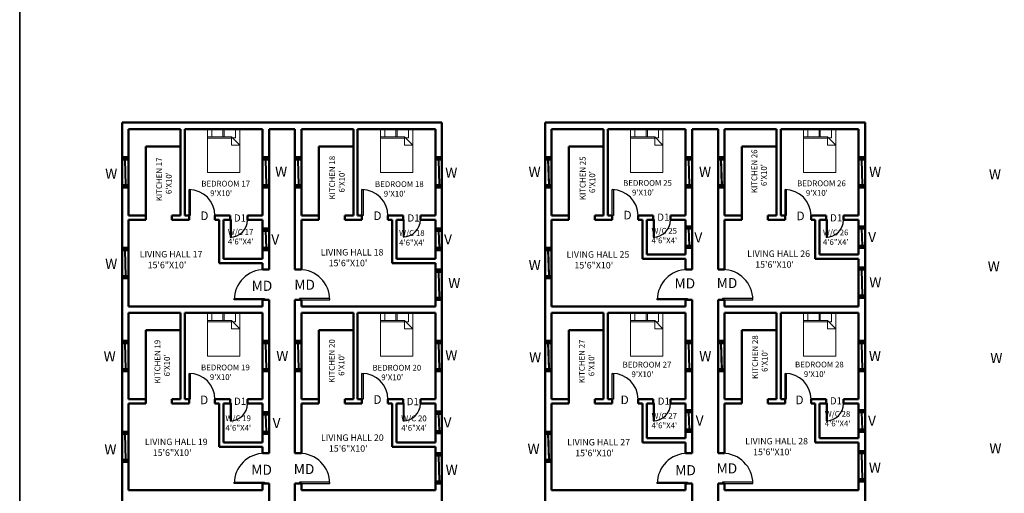
# Model space of a CAD drawing. Units: inches. Extents: x 9239 to 26065, y 6728 to 14611.
# Tile 8 of 12: x 23324 to 24691, y 12444 to 13102. Entities that reach past the tile are written whole.
import ezdxf

# ---------------------------------------------------------------- set-up
doc = ezdxf.new("R2010")
doc.units = ezdxf.units.IN
doc.header["$MEASUREMENT"] = 0
for name, color, linetype, lineweight in [('A-ANNO-TEXT', 7, 'Continuous', 18), ('A-ANNO-TTLB', 7, 'Continuous', 35), ('A-AREA-IDEN', 7, 'Continuous', 18), ('A-DOOR', 4, 'Continuous', 25), ('A-FURN', 8, 'Continuous', 18), ('A-GLAZ', 4, 'Continuous', 25), ('A-WALL', 7, 'Continuous', 50)]:
    doc.layers.add(name, color=color, linetype=linetype, lineweight=lineweight)
doc.styles.get("Standard").update_dxf_attribs({"font": 'arial.ttf'})

# ---------------------------------------------------------------- blocks, each defined once
blk = doc.blocks.new('*U10')
for p, q in [((0, 0), (0, -6)), ((36, 0), (36, -6))]:
    blk.add_line(p, q)
blk.add_lwpolyline([(0, 0), (0, 36), (1.75, 36), (1.75, 0)], close=True)
blk.add_arc((0, 0), 36, 0, 90)
blk = doc.blocks.new('*U34')
for p, q in [((0, 0), (0, 6)), ((24, 0), (24, 6))]:
    blk.add_line(p, q)
blk.add_lwpolyline([(0, 0), (0, -24), (1.75, -24), (1.75, 0)], close=True)
blk.add_arc((0, 0), 24, 270, 0)
blk = doc.blocks.new('*U33')
for p, q in [((-40, 0), (-40, 6)), ((0, 0), (0, 6))]:
    blk.add_line(p, q)
blk.add_lwpolyline([(0, 0), (0, -40), (-1.75, -40), (-1.75, 0)], close=True)
blk.add_arc((0, 0), 40, 180, 270)
blk = doc.blocks.new('*U35')
for p, q in [((0, 0), (0, -6)), ((-40, 0), (-40, -6))]:
    blk.add_line(p, q)
blk.add_lwpolyline([(0, 0), (0, 40), (-1.75, 40), (-1.75, 0)], close=True)
blk.add_arc((0, 0), 40, 90, 180)
blk = doc.blocks.new('Bed - Queen')
for p, q in [((0, -80.00003), (0, 0)), ((0, 0), (59.99999, 0)), ((59.99999, 0), (59.99999, -80.00003)), ((0, -14.4), (44.8, -14.4)), ((44.8, -16.8), (0, -16.8)), ((7.99999, -1.2), (28.79998, -1.2)), ((7.99999, -14.4), (7.99999, -1.2)), ((28.79998, -1.2), (28.79998, -14.4)), ((31.19999, -1.2), (51.99999, -1.2)), ((31.19999, -14.4), (31.19999, -1.2)), ((59.99999, -29.6), (44.8, -14.4)), ((44.8, -14.4), (44.8, -29.6)), ((51.99999, -16.4), (46.79936, -16.4)), ((51.99999, -1.2), (51.99999, -16.4)), ((44.8, -29.6), (59.99999, -29.6)), ((59.99999, -80.00003), (0, -80.00003))]:
    blk.add_line(p, q)
blk = doc.blocks.new('WIN-36')
for p, q in [((0, 1), (36, 1)), ((0, 0.5), (36, 0.5)), ((0, 0), (36, 0))]:
    blk.add_line(p, q)
blk = doc.blocks.new('WIN-24')
for p, q in [((0, 1), (24, 1)), ((0, 0.5), (24, 0.5)), ((0, 0), (24, 0))]:
    blk.add_line(p, q)

msp = doc.modelspace()

# ---------------------------------------------------------------- linework, layer by layer
at = {"layer": 'A-ANNO-TTLB'}
msp.add_lwpolyline([(23324.14, 14611.25), (26064.6, 14611.25), (26064.6, 11591.84), (23324.14, 11591.84)], close=True, dxfattribs=at)
at = {"layer": 'A-WALL'}
for p, q in [((23466.16, 12958.64), (23910.16, 12958.64)), ((23466.16, 11854.64), (23466.16, 12958.64)), ((23910.16, 12958.64), (23910.16, 11854.64)), ((24053.28, 12958.64), (24497.28, 12958.64)), ((24053.28, 11854.64), (24053.28, 12958.64)), ((24497.28, 12958.64), (24497.28, 11854.64)), ((23475.16, 12949.64), (23547.16, 12949.64)), ((23475.16, 12829.64), (23475.16, 12949.64)), ((23547.16, 12829.64), (23547.16, 12949.64)), ((23553.16, 12829.64), (23553.16, 12949.64)), ((23553.16, 12949.64), (23661.16, 12949.64)), ((23661.16, 12829.64), (23661.16, 12949.64)), ((23670.16, 12754.64), (23670.16, 12949.64)), ((23670.16, 12949.64), (23706.16, 12949.64)), ((23706.16, 12949.64), (23706.16, 12754.64)), ((23715.16, 12949.64), (23715.16, 12829.64)), ((23715.16, 12949.64), (23787.16, 12949.64)), ((23787.16, 12949.64), (23787.16, 12829.64)), ((23793.16, 12949.64), (23793.16, 12829.64)), ((23793.16, 12949.64), (23901.16, 12949.64)), ((23901.16, 12949.64), (23901.16, 12829.64)), ((24062.28, 12949.64), (24134.28, 12949.64)), ((24062.28, 12829.64), (24062.28, 12949.64)), ((24134.28, 12829.64), (24134.28, 12949.64)), ((24140.28, 12829.64), (24140.28, 12949.64)), ((24140.28, 12949.64), (24248.28, 12949.64)), ((24248.28, 12829.64), (24248.28, 12949.64)), ((24257.28, 12754.64), (24257.28, 12949.64)), ((24257.28, 12949.64), (24293.28, 12949.64)), ((24293.28, 12949.64), (24293.28, 12754.64)), ((24302.28, 12949.64), (24302.28, 12829.64)), ((24302.28, 12949.64), (24374.28, 12949.64)), ((24374.28, 12949.64), (24374.28, 12829.64)), ((24380.28, 12949.64), (24380.28, 12829.64)), ((24380.28, 12949.64), (24488.28, 12949.64)), ((24488.28, 12949.64), (24488.28, 12829.64)), ((23499.16, 12829.64), (23499.16, 12925.64)), ((23499.16, 12925.64), (23547.16, 12925.64)), ((23739.16, 12925.64), (23739.16, 12829.64)), ((23739.16, 12925.64), (23787.16, 12925.64)), ((24086.28, 12829.64), (24086.28, 12925.64)), ((24086.28, 12925.64), (24134.28, 12925.64)), ((24326.28, 12925.64), (24326.28, 12829.64)), ((24326.28, 12925.64), (24374.28, 12925.64)), ((23475.16, 12910.64), (23466.16, 12910.64)), ((23475.16, 12907.64), (23466.16, 12907.64)), ((23661.16, 12910.64), (23670.16, 12910.64)), ((23661.16, 12907.64), (23670.16, 12907.64)), ((23715.16, 12910.64), (23706.16, 12910.64)), ((23715.16, 12907.64), (23706.16, 12907.64)), ((23901.16, 12910.64), (23910.16, 12910.64)), ((23901.16, 12907.64), (23910.16, 12907.64)), ((24062.28, 12910.64), (24053.28, 12910.64)), ((24062.28, 12907.64), (24053.28, 12907.64)), ((24248.28, 12910.64), (24257.28, 12910.64)), ((24248.28, 12907.64), (24257.28, 12907.64)), ((24302.28, 12910.64), (24293.28, 12910.64)), ((24302.28, 12907.64), (24293.28, 12907.64)), ((24488.28, 12910.64), (24497.28, 12910.64)), ((24488.28, 12907.64), (24497.28, 12907.64)), ((23475.16, 12871.64), (23466.16, 12871.64)), ((23661.16, 12871.64), (23670.16, 12871.64)), ((23715.16, 12871.64), (23706.16, 12871.64)), ((23901.16, 12871.64), (23910.16, 12871.64)), ((24062.28, 12871.64), (24053.28, 12871.64)), ((24248.28, 12871.64), (24257.28, 12871.64)), ((24302.28, 12871.64), (24293.28, 12871.64)), ((24488.28, 12871.64), (24497.28, 12871.64)), ((23475.16, 12868.64), (23466.16, 12868.64)), ((23661.16, 12868.64), (23670.16, 12868.64)), ((23715.16, 12868.64), (23706.16, 12868.64)), ((23901.16, 12868.64), (23910.16, 12868.64)), ((24062.28, 12868.64), (24053.28, 12868.64)), ((24248.28, 12868.64), (24257.28, 12868.64)), ((24302.28, 12868.64), (24293.28, 12868.64)), ((24488.28, 12868.64), (24497.28, 12868.64)), ((23475.16, 12829.64), (23499.16, 12829.64)), ((23475.16, 12823.64), (23499.16, 12823.64)), ((23475.16, 12703.64), (23475.16, 12823.64)), ((23499.16, 12823.64), (23499.16, 12829.64)), ((23535.16, 12823.64), (23535.16, 12829.64)), ((23535.16, 12829.64), (23547.16, 12829.64)), ((23535.16, 12823.64), (23559.16, 12823.64)), ((23553.16, 12829.64), (23559.16, 12829.64)), ((23559.16, 12823.64), (23559.16, 12829.64)), ((23595.16, 12823.64), (23595.16, 12829.64)), ((23595.16, 12829.64), (23616.16, 12829.64)), ((23595.16, 12823.64), (23601.16, 12823.64)), ((23601.16, 12763.64), (23601.16, 12823.64)), ((23607.16, 12769.64), (23607.16, 12823.64)), ((23607.16, 12823.64), (23616.16, 12823.64)), ((23616.16, 12823.64), (23616.16, 12829.64)), ((23640.16, 12823.64), (23640.16, 12829.64)), ((23640.16, 12829.64), (23661.16, 12829.64)), ((23640.16, 12823.64), (23661.16, 12823.64)), ((23661.16, 12769.64), (23661.16, 12823.64)), ((23715.16, 12829.64), (23739.16, 12829.64)), ((23715.16, 12823.64), (23739.16, 12823.64)), ((23715.16, 12823.64), (23715.16, 12754.64)), ((23739.16, 12829.64), (23739.16, 12823.64)), ((23775.16, 12829.64), (23775.16, 12823.64)), ((23775.16, 12829.64), (23787.16, 12829.64)), ((23775.16, 12823.64), (23799.16, 12823.64)), ((23793.16, 12829.64), (23799.16, 12829.64)), ((23799.16, 12829.64), (23799.16, 12823.64)), ((23835.16, 12829.64), (23835.16, 12823.64)), ((23835.16, 12829.64), (23856.16, 12829.64)), ((23835.16, 12823.64), (23841.16, 12823.64)), ((23841.16, 12823.64), (23841.16, 12763.64)), ((23847.16, 12823.64), (23847.16, 12769.64)), ((23847.16, 12823.64), (23856.16, 12823.64)), ((23856.16, 12829.64), (23856.16, 12823.64)), ((23880.16, 12829.64), (23880.16, 12823.64)), ((23880.16, 12829.64), (23901.16, 12829.64)), ((23880.16, 12823.64), (23901.16, 12823.64)), ((23901.16, 12823.64), (23901.16, 12769.64)), ((24062.28, 12829.64), (24086.28, 12829.64)), ((24062.28, 12823.64), (24086.28, 12823.64)), ((24062.28, 12703.64), (24062.28, 12823.64)), ((24086.28, 12823.64), (24086.28, 12829.64)), ((24122.28, 12823.64), (24122.28, 12829.64)), ((24122.28, 12829.64), (24134.28, 12829.64)), ((24122.28, 12823.64), (24146.28, 12823.64)), ((24140.28, 12829.64), (24146.28, 12829.64)), ((24146.28, 12823.64), (24146.28, 12829.64)), ((24182.28, 12823.64), (24182.28, 12829.64)), ((24182.28, 12829.64), (24203.28, 12829.64)), ((24182.28, 12823.64), (24188.28, 12823.64)), ((24188.28, 12769.64), (24188.28, 12823.64)), ((24194.28, 12775.64), (24194.28, 12823.64)), ((24194.28, 12823.64), (24203.28, 12823.64)), ((24203.28, 12823.64), (24203.28, 12829.64)), ((24227.28, 12823.64), (24227.28, 12829.64)), ((24227.28, 12829.64), (24248.28, 12829.64)), ((24227.28, 12823.64), (24248.28, 12823.64)), ((24248.28, 12775.64), (24248.28, 12823.64)), ((24302.28, 12829.64), (24326.28, 12829.64)), ((24302.28, 12823.64), (24326.28, 12823.64)), ((24302.28, 12823.64), (24302.28, 12754.64)), ((24326.28, 12829.64), (24326.28, 12823.64)), ((24362.28, 12829.64), (24362.28, 12823.64)), ((24362.28, 12829.64), (24374.28, 12829.64)), ((24362.28, 12823.64), (24386.28, 12823.64)), ((24380.28, 12829.64), (24386.28, 12829.64)), ((24386.28, 12829.64), (24386.28, 12823.64)), ((24422.28, 12829.64), (24422.28, 12823.64)), ((24422.28, 12829.64), (24443.28, 12829.64)), ((24422.28, 12823.64), (24428.28, 12823.64)), ((24428.28, 12823.64), (24428.28, 12769.64)), ((24434.28, 12823.64), (24434.28, 12775.64)), ((24434.28, 12823.64), (24443.28, 12823.64)), ((24443.28, 12829.64), (24443.28, 12823.64)), ((24467.28, 12829.64), (24467.28, 12823.64)), ((24467.28, 12829.64), (24488.28, 12829.64)), ((24467.28, 12823.64), (24488.28, 12823.64)), ((24488.28, 12823.64), (24488.28, 12775.64)), ((23661.16, 12811.64), (23670.16, 12811.64)), ((23661.16, 12808.64), (23670.16, 12808.64)), ((23901.16, 12811.64), (23910.16, 12811.64)), ((23901.16, 12808.64), (23910.16, 12808.64)), ((24248.28, 12814.64), (24257.28, 12814.64)), ((24248.28, 12811.64), (24257.28, 12811.64)), ((24488.28, 12814.64), (24497.28, 12814.64)), ((24488.28, 12811.64), (24497.28, 12811.64)), ((23475.16, 12784.64), (23466.16, 12784.64)), ((23475.16, 12781.64), (23466.16, 12781.64)), ((23661.16, 12784.64), (23670.16, 12784.64)), ((23661.16, 12781.64), (23670.16, 12781.64)), ((23901.16, 12784.64), (23910.16, 12784.64)), ((23901.16, 12781.64), (23910.16, 12781.64)), ((24062.28, 12784.64), (24053.28, 12784.64)), ((24062.28, 12781.64), (24053.28, 12781.64)), ((24248.28, 12787.64), (24257.28, 12787.64)), ((24248.28, 12784.64), (24257.28, 12784.64)), ((24488.28, 12787.64), (24497.28, 12787.64)), ((24488.28, 12784.64), (24497.28, 12784.64)), ((23601.16, 12763.64), (23661.16, 12763.64)), ((23607.16, 12769.64), (23661.16, 12769.64)), ((23661.16, 12754.64), (23661.16, 12763.64)), ((23841.16, 12763.64), (23901.16, 12763.64)), ((23847.16, 12769.64), (23901.16, 12769.64)), ((23901.16, 12763.64), (23901.16, 12703.64)), ((24188.28, 12769.64), (24248.28, 12769.64)), ((24194.28, 12775.64), (24248.28, 12775.64)), ((24248.28, 12754.64), (24248.28, 12769.64)), ((24428.28, 12769.64), (24488.28, 12769.64)), ((24434.28, 12775.64), (24488.28, 12775.64)), ((24488.28, 12769.64), (24488.28, 12703.64)), ((23661.16, 12754.64), (23670.16, 12754.64)), ((23706.16, 12754.64), (23715.16, 12754.64)), ((23901.16, 12754.64), (23910.16, 12754.64)), ((23901.16, 12751.64), (23910.16, 12751.64)), ((24248.28, 12754.64), (24257.28, 12754.64)), ((24293.28, 12754.64), (24302.28, 12754.64)), ((24488.28, 12757.64), (24497.28, 12757.64)), ((24488.28, 12754.64), (24497.28, 12754.64)), ((23475.16, 12745.64), (23466.16, 12745.64)), ((23475.16, 12742.64), (23466.16, 12742.64)), ((24062.28, 12745.64), (24053.28, 12745.64)), ((24062.28, 12742.64), (24053.28, 12742.64)), ((23661.16, 12712.64), (23670.16, 12712.64)), ((23661.16, 12703.64), (23661.16, 12712.64)), ((23670.16, 12499.64), (23670.16, 12712.64)), ((23706.16, 12712.64), (23715.16, 12712.64)), ((23706.16, 12712.64), (23706.16, 12499.64)), ((23715.16, 12712.64), (23715.16, 12703.64)), ((23901.16, 12715.64), (23910.16, 12715.64)), ((23901.16, 12712.64), (23910.16, 12712.64)), ((24248.28, 12712.64), (24257.28, 12712.64)), ((24248.28, 12703.64), (24248.28, 12712.64)), ((24257.28, 12499.64), (24257.28, 12712.64)), ((24293.28, 12712.64), (24302.28, 12712.64)), ((24293.28, 12712.64), (24293.28, 12499.64)), ((24302.28, 12712.64), (24302.28, 12703.64)), ((24488.28, 12718.64), (24497.28, 12718.64)), ((24488.28, 12715.64), (24497.28, 12715.64)), ((23475.16, 12703.64), (23661.16, 12703.64)), ((23475.16, 12694.64), (23547.16, 12694.64)), ((23475.16, 12574.64), (23475.16, 12694.64)), ((23547.16, 12574.64), (23547.16, 12694.64)), ((23553.16, 12574.64), (23553.16, 12694.64)), ((23553.16, 12694.64), (23661.16, 12694.64)), ((23661.16, 12574.64), (23661.16, 12694.64)), ((23715.16, 12703.64), (23901.16, 12703.64)), ((23715.16, 12694.64), (23787.16, 12694.64)), ((23715.16, 12694.64), (23715.16, 12574.64)), ((23787.16, 12694.64), (23787.16, 12574.64)), ((23793.16, 12694.64), (23793.16, 12574.64)), ((23793.16, 12694.64), (23901.16, 12694.64)), ((23901.16, 12694.64), (23901.16, 12574.64)), ((24062.28, 12703.64), (24248.28, 12703.64)), ((24062.28, 12694.64), (24134.28, 12694.64)), ((24062.28, 12574.64), (24062.28, 12694.64)), ((24134.28, 12574.64), (24134.28, 12694.64)), ((24140.28, 12574.64), (24140.28, 12694.64)), ((24140.28, 12694.64), (24248.28, 12694.64)), ((24248.28, 12574.64), (24248.28, 12694.64)), ((24302.28, 12703.64), (24488.28, 12703.64)), ((24302.28, 12694.64), (24374.28, 12694.64)), ((24302.28, 12694.64), (24302.28, 12574.64)), ((24374.28, 12694.64), (24374.28, 12574.64)), ((24380.28, 12694.64), (24380.28, 12574.64)), ((24380.28, 12694.64), (24488.28, 12694.64)), ((24488.28, 12694.64), (24488.28, 12574.64)), ((23499.16, 12574.64), (23499.16, 12670.64)), ((23499.16, 12670.64), (23547.16, 12670.64)), ((23739.16, 12670.64), (23739.16, 12574.64)), ((23739.16, 12670.64), (23787.16, 12670.64)), ((24086.28, 12574.64), (24086.28, 12670.64)), ((24086.28, 12670.64), (24134.28, 12670.64)), ((24326.28, 12670.64), (24326.28, 12574.64)), ((24326.28, 12670.64), (24374.28, 12670.64)), ((23475.16, 12655.64), (23466.16, 12655.64)), ((23661.16, 12655.64), (23670.16, 12655.64)), ((23715.16, 12655.64), (23706.16, 12655.64)), ((23901.16, 12655.64), (23910.16, 12655.64)), ((24062.28, 12655.64), (24053.28, 12655.64)), ((24248.28, 12655.64), (24257.28, 12655.64)), ((24302.28, 12655.64), (24293.28, 12655.64)), ((24488.28, 12655.64), (24497.28, 12655.64)), ((23475.16, 12652.64), (23466.16, 12652.64)), ((23661.16, 12652.64), (23670.16, 12652.64)), ((23715.16, 12652.64), (23706.16, 12652.64)), ((23901.16, 12652.64), (23910.16, 12652.64)), ((24062.28, 12652.64), (24053.28, 12652.64)), ((24248.28, 12652.64), (24257.28, 12652.64)), ((24302.28, 12652.64), (24293.28, 12652.64)), ((24488.28, 12652.64), (24497.28, 12652.64)), ((23475.16, 12616.64), (23466.16, 12616.64)), ((23475.16, 12613.64), (23466.16, 12613.64)), ((23661.16, 12616.64), (23670.16, 12616.64)), ((23661.16, 12613.64), (23670.16, 12613.64)), ((23715.16, 12616.64), (23706.16, 12616.64)), ((23715.16, 12613.64), (23706.16, 12613.64)), ((23901.16, 12616.64), (23910.16, 12616.64)), ((23901.16, 12613.64), (23910.16, 12613.64)), ((24062.28, 12616.64), (24053.28, 12616.64)), ((24062.28, 12613.64), (24053.28, 12613.64)), ((24248.28, 12616.64), (24257.28, 12616.64)), ((24248.28, 12613.64), (24257.28, 12613.64)), ((24302.28, 12616.64), (24293.28, 12616.64)), ((24302.28, 12613.64), (24293.28, 12613.64)), ((24488.28, 12616.64), (24497.28, 12616.64)), ((24488.28, 12613.64), (24497.28, 12613.64)), ((23475.16, 12574.64), (23499.16, 12574.64)), ((23499.16, 12568.64), (23499.16, 12574.64)), ((23535.16, 12568.64), (23535.16, 12574.64)), ((23535.16, 12574.64), (23547.16, 12574.64)), ((23553.16, 12574.64), (23559.16, 12574.64)), ((23559.16, 12568.64), (23559.16, 12574.64)), ((23595.16, 12568.64), (23595.16, 12574.64)), ((23595.16, 12574.64), (23616.16, 12574.64)), ((23616.16, 12568.64), (23616.16, 12574.64)), ((23640.16, 12568.64), (23640.16, 12574.64)), ((23640.16, 12574.64), (23661.16, 12574.64)), ((23715.16, 12574.64), (23739.16, 12574.64)), ((23739.16, 12574.64), (23739.16, 12568.64)), ((23775.16, 12574.64), (23775.16, 12568.64)), ((23775.16, 12574.64), (23787.16, 12574.64)), ((23793.16, 12574.64), (23799.16, 12574.64)), ((23799.16, 12574.64), (23799.16, 12568.64)), ((23835.16, 12574.64), (23835.16, 12568.64)), ((23835.16, 12574.64), (23856.16, 12574.64)), ((23856.16, 12574.64), (23856.16, 12568.64)), ((23880.16, 12574.64), (23880.16, 12568.64)), ((23880.16, 12574.64), (23901.16, 12574.64)), ((24062.28, 12574.64), (24086.28, 12574.64)), ((24086.28, 12568.64), (24086.28, 12574.64)), ((24122.28, 12568.64), (24122.28, 12574.64)), ((24122.28, 12574.64), (24134.28, 12574.64)), ((24140.28, 12574.64), (24146.28, 12574.64)), ((24146.28, 12568.64), (24146.28, 12574.64)), ((24182.28, 12568.64), (24182.28, 12574.64)), ((24182.28, 12574.64), (24203.28, 12574.64)), ((24203.28, 12568.64), (24203.28, 12574.64)), ((24227.28, 12568.64), (24227.28, 12574.64)), ((24227.28, 12574.64), (24248.28, 12574.64)), ((24302.28, 12574.64), (24326.28, 12574.64)), ((24326.28, 12574.64), (24326.28, 12568.64)), ((24362.28, 12574.64), (24362.28, 12568.64)), ((24362.28, 12574.64), (24374.28, 12574.64)), ((24380.28, 12574.64), (24386.28, 12574.64)), ((24386.28, 12574.64), (24386.28, 12568.64)), ((24422.28, 12574.64), (24422.28, 12568.64)), ((24422.28, 12574.64), (24443.28, 12574.64)), ((24443.28, 12574.64), (24443.28, 12568.64)), ((24467.28, 12574.64), (24467.28, 12568.64)), ((24467.28, 12574.64), (24488.28, 12574.64)), ((23475.16, 12568.64), (23499.16, 12568.64)), ((23475.16, 12448.64), (23475.16, 12568.64)), ((23535.16, 12568.64), (23559.16, 12568.64)), ((23595.16, 12568.64), (23601.16, 12568.64)), ((23601.16, 12508.64), (23601.16, 12568.64)), ((23607.16, 12514.64), (23607.16, 12568.64)), ((23607.16, 12568.64), (23616.16, 12568.64)), ((23640.16, 12568.64), (23661.16, 12568.64)), ((23661.16, 12514.64), (23661.16, 12568.64)), ((23715.16, 12568.64), (23739.16, 12568.64)), ((23715.16, 12568.64), (23715.16, 12499.64)), ((23775.16, 12568.64), (23799.16, 12568.64)), ((23835.16, 12568.64), (23841.16, 12568.64)), ((23841.16, 12568.64), (23841.16, 12508.64)), ((23847.16, 12568.64), (23847.16, 12514.64)), ((23847.16, 12568.64), (23856.16, 12568.64)), ((23880.16, 12568.64), (23901.16, 12568.64)), ((23901.16, 12568.64), (23901.16, 12514.64)), ((23901.16, 12557.55), (23910.16, 12557.55)), ((24062.28, 12568.64), (24086.28, 12568.64)), ((24062.28, 12448.64), (24062.28, 12568.64)), ((24122.28, 12568.64), (24146.28, 12568.64)), ((24182.28, 12568.64), (24188.28, 12568.64)), ((24188.28, 12514.64), (24188.28, 12568.64)), ((24194.28, 12520.64), (24194.28, 12568.64)), ((24194.28, 12568.64), (24203.28, 12568.64)), ((24227.28, 12568.64), (24248.28, 12568.64)), ((24248.28, 12520.64), (24248.28, 12568.64)), ((24248.28, 12559.64), (24257.28, 12559.64)), ((24302.28, 12568.64), (24326.28, 12568.64)), ((24302.28, 12568.64), (24302.28, 12499.64)), ((24362.28, 12568.64), (24386.28, 12568.64)), ((24422.28, 12568.64), (24428.28, 12568.64)), ((24428.28, 12568.64), (24428.28, 12514.64)), ((24434.28, 12568.64), (24434.28, 12520.64)), ((24434.28, 12568.64), (24443.28, 12568.64)), ((24467.28, 12568.64), (24488.28, 12568.64)), ((24488.28, 12568.64), (24488.28, 12520.64)), ((24488.28, 12559.64), (24497.28, 12559.64)), ((23661.16, 12556.64), (23670.16, 12556.64)), ((23661.16, 12553.64), (23670.16, 12553.64)), ((23901.16, 12554.55), (23910.16, 12554.55)), ((24248.28, 12556.64), (24257.28, 12556.64)), ((24488.28, 12556.64), (24497.28, 12556.64)), ((23901.16, 12530.55), (23910.16, 12530.55)), ((24248.28, 12532.64), (24257.28, 12532.64)), ((24488.28, 12532.64), (24497.28, 12532.64)), ((23475.16, 12529.64), (23466.16, 12529.64)), ((23475.16, 12526.64), (23466.16, 12526.64)), ((23661.16, 12529.64), (23670.16, 12529.64)), ((23661.16, 12526.64), (23670.16, 12526.64)), ((23901.16, 12527.55), (23910.16, 12527.55)), ((24062.28, 12529.64), (24053.28, 12529.64)), ((24062.28, 12526.64), (24053.28, 12526.64)), ((24194.28, 12520.64), (24248.28, 12520.64)), ((24248.28, 12529.64), (24257.28, 12529.64)), ((24434.28, 12520.64), (24488.28, 12520.64)), ((24488.28, 12529.64), (24497.28, 12529.64)), ((23601.16, 12508.64), (23661.16, 12508.64)), ((23607.16, 12514.64), (23661.16, 12514.64)), ((23661.16, 12499.64), (23661.16, 12508.64)), ((23841.16, 12508.64), (23901.16, 12508.64)), ((23847.16, 12514.64), (23901.16, 12514.64)), ((23901.16, 12508.64), (23901.16, 12448.64)), ((24188.28, 12514.64), (24248.28, 12514.64)), ((24248.28, 12499.64), (24248.28, 12514.64)), ((24428.28, 12514.64), (24488.28, 12514.64)), ((24488.28, 12514.64), (24488.28, 12448.64)), ((24488.28, 12502.64), (24497.28, 12502.64)), ((23475.16, 12490.64), (23466.16, 12490.64)), ((23661.16, 12499.64), (23670.16, 12499.64)), ((23706.16, 12499.64), (23715.16, 12499.64)), ((23901.16, 12499.64), (23910.16, 12499.64)), ((23901.16, 12496.64), (23910.16, 12496.64)), ((24062.28, 12490.64), (24053.28, 12490.64)), ((24248.28, 12499.64), (24257.28, 12499.64)), ((24293.28, 12499.64), (24302.28, 12499.64)), ((24488.28, 12499.64), (24497.28, 12499.64)), ((23475.16, 12487.64), (23466.16, 12487.64)), ((24062.28, 12487.64), (24053.28, 12487.64)), ((24488.28, 12463.64), (24497.28, 12463.64)), ((23475.16, 12448.64), (23661.16, 12448.64)), ((23661.16, 12457.64), (23670.16, 12457.64)), ((23661.16, 12448.64), (23661.16, 12457.64)), ((23670.16, 12244.64), (23670.16, 12457.64)), ((23706.16, 12457.64), (23715.16, 12457.64)), ((23706.16, 12457.64), (23706.16, 12244.64)), ((23715.16, 12457.64), (23715.16, 12448.64)), ((23715.16, 12448.64), (23901.16, 12448.64)), ((23901.16, 12460.64), (23910.16, 12460.64)), ((23901.16, 12457.64), (23910.16, 12457.64)), ((24062.28, 12448.64), (24248.28, 12448.64)), ((24248.28, 12457.64), (24257.28, 12457.64)), ((24248.28, 12448.64), (24248.28, 12457.64)), ((24257.28, 12244.64), (24257.28, 12457.64)), ((24293.28, 12457.64), (24302.28, 12457.64)), ((24293.28, 12457.64), (24293.28, 12244.64)), ((24302.28, 12457.64), (24302.28, 12448.64)), ((24302.28, 12448.64), (24488.28, 12448.64)), ((24488.28, 12460.64), (24497.28, 12460.64))]:
    msp.add_line(p, q, dxfattribs=at)

# ---------------------------------------------------------------- block references
at = {"layer": 'A-DOOR'}
for name, p in [('*U10', (23559.16, 12829.64)), ('*U10', (23799.16, 12829.64)), ('*U10', (24146.28, 12829.64)), ('*U10', (24386.28, 12829.64)), ('*U34', (23616.16, 12823.64)), ('*U34', (23856.16, 12823.97)), ('*U34', (24203.28, 12823.64)), ('*U34', (24443.28, 12823.64)), ('*U10', (23559.16, 12574.64)), ('*U10', (23799.16, 12574.64)), ('*U10', (24146.28, 12574.64)), ('*U10', (24386.28, 12574.64)), ('*U34', (23616.16, 12568.64)), ('*U34', (23856.16, 12568.64)), ('*U34', (24203.28, 12568.64)), ('*U34', (24443.28, 12568.64))]:
    msp.add_blockref(name, p, dxfattribs=at)
at = {"layer": 'A-DOOR', "rotation": 270}
for name, p, xscale, yscale, zscale in [('*U33', (23663.86, 12712.64), 1.05, 1.05, 1.05), ('*U35', (23712.46, 12712.64), 1.05, 1.05, 1.05), ('*U33', (24250.98, 12712.64), 1.050020150174431, 1.050020150174431, 1.050020150174431), ('*U35', (24299.58, 12712.64), 1.05, 1.05, 1.05), ('*U33', (23663.86, 12457.64), 1.049999999999956, 1.049999999999956, 1.049999999999956), ('*U35', (23712.46, 12457.64), 1.05, 1.05, 1.05), ('*U33', (24250.98, 12457.64), 1.05, 1.05, 1.05), ('*U35', (24299.58, 12457.64), 1.05, 1.05, 1.05)]:
    msp.add_blockref(name, p, dxfattribs=dict(at, xscale=xscale, yscale=yscale, zscale=zscale))
at = {"layer": 'A-FURN', "xscale": 0.75, "yscale": 0.75, "zscale": 0.75}
for p in [(23584.66, 12949.64), (23824.66, 12949.64), (24171.78, 12949.64), (24411.78, 12949.64), (23584.66, 12694.64), (23824.66, 12694.64), (24171.78, 12694.64), (24411.78, 12694.64)]:
    msp.add_blockref('Bed - Queen', p, dxfattribs=at)
at = {"layer": 'A-GLAZ'}
for name, p, rotation in [('WIN-36', (23469.66, 12907.62), 271.5911402711888), ('WIN-36', (23664.66, 12907.62), 271.5911402712119), ('WIN-36', (23709.66, 12907.62), 271.5911402711888), ('WIN-36', (23904.66, 12907.62), 271.5911402711888), ('WIN-36', (24056.78, 12907.62), 271.5911402712003), ('WIN-36', (24251.78, 12907.62), 271.5911402712003), ('WIN-36', (24296.78, 12907.62), 271.5911402711656), ('WIN-36', (24491.78, 12907.62), 271.5911402712003), ('WIN-24', (23664.66, 12808.61), 272.3859440303801), ('WIN-24', (23904.66, 12808.61), 272.3859440304149), ('WIN-24', (24251.78, 12811.61), 272.3859440303975), ('WIN-24', (24491.78, 12811.61), 272.3859440303975), ('WIN-36', (23469.66, 12781.62), 271.5911402712003), ('WIN-36', (24056.78, 12781.62), 271.5911402711772), ('WIN-36', (23904.66, 12751.62), 271.5911402712119), ('WIN-36', (24491.78, 12754.62), 271.5911402712003), ('WIN-36', (23469.66, 12652.62), 271.5911402711888), ('WIN-36', (23664.66, 12652.62), 271.5911402711888), ('WIN-36', (23709.66, 12652.62), 271.5911402712003), ('WIN-36', (23904.66, 12652.62), 271.5911402712119), ('WIN-36', (24056.78, 12652.62), 271.5911402711656), ('WIN-36', (24251.78, 12652.62), 271.5911402712003), ('WIN-36', (24296.78, 12652.62), 271.5911402712003), ('WIN-36', (24491.78, 12652.62), 271.5911402712003), ('WIN-24', (23664.66, 12553.61), 272.3859440303801), ('WIN-24', (23904.66, 12554.51), 272.3859440303801), ('WIN-24', (24251.78, 12556.61), 272.3859440303975), ('WIN-24', (24491.78, 12556.61), 272.3859440303975), ('WIN-36', (23469.66, 12526.62), 271.5911402712003), ('WIN-36', (24056.78, 12526.62), 271.5911402712003), ('WIN-36', (23904.66, 12496.62), 271.5911402711888), ('WIN-36', (24491.78, 12499.62), 271.5911402712003)]:
    msp.add_blockref(name, p, dxfattribs=dict(at, rotation=rotation))

# ---------------------------------------------------------------- texts
at = {"layer": 'A-ANNO-TEXT', "attachment_point": 1}
for s, width, insert, char_height in [('W', 545.3335, (23442.82, 12894.78), 14), ('W', 545.3335, (23678.59, 12897.72), 14), ('W', 545.3335, (23914.71, 12896.24), 14), ('W', 545.3335, (24030.29, 12897.33), 14), ('W', 545.3335, (24266.85, 12897.37), 14), ('W', 545.3335, (24502.94, 12897.39), 14), ('W', 545.3335, (24669.17, 12893.98), 14), ('D', 545.3335, (23574.81, 12835.36), 12), ('D1', 545.3335, (23621.38, 12831.3), 10), ('D', 545.3335, (23815, 12835.47), 12), ('D1', 545.3335, (23862.23, 12831.32), 10), ('D', 545.3335, (24162.05, 12836.3), 12), ('D1', 545.3335, (24208.92, 12832.45), 10), ('D', 545.3335, (24402.14, 12835.16), 12), ('D1', 545.3335, (24448.71, 12831.51), 10), ('W/C 17\\P4\'6"X4\'', 1026.6179, (23613.01, 12810.91), 8), ('V', 545.3335, (23673.28, 12803.49), 14), ('W/C 18\\P4\'6"X4\'', 1026.6179, (23850.68, 12809.44), 8), ('V', 545.3335, (23913.06, 12803.71), 14), ('W/C 25\\P4\'6"X4\'', 1026.6179, (24200.93, 12812.49), 8), ('V', 545.3335, (24260.44, 12806.3), 14), ('W/C 26\\P4\'6"X4\'', 1026.6179, (24438.83, 12810.19), 8), ('V', 545.3335, (24501.62, 12806.95), 14), ('W', 545.3335, (23442.81, 12769.67), 14), ('W', 545.3335, (24030.46, 12767.91), 14), ('W', 545.3335, (24667.49, 12766.16), 14), ('MD', 545.3335, (23646.03, 12739.17), 14), ('MD', 545.3335, (23705.25, 12740.65), 14), ('W', 545.3335, (23918.89, 12742.94), 14), ('MD', 545.3335, (24232.87, 12742.51), 14), ('MD', 545.3335, (24291.38, 12743), 14), ('W', 545.3335, (24503.2, 12743.95), 14), ('W', 545.3335, (23440.61, 12641.22), 14), ('W', 545.3335, (23680.21, 12641.88), 14), ('W', 545.3335, (23914.77, 12642.82), 14), ('W', 545.3335, (24031.15, 12639.99), 14), ('W', 545.3335, (24267.17, 12641.46), 14), ('W', 545.3335, (24502.61, 12641.71), 14), ('W', 545.3335, (24671.13, 12638.99), 14), ('D', 545.3335, (23574.53, 12579.8), 12), ('D1', 545.3335, (23621.55, 12576.89), 10), ('D', 545.3335, (23815, 12580.31), 12), ('D1', 545.3335, (23861.18, 12576.44), 10), ('D', 545.3335, (24158.08, 12579.89), 12), ('D1', 545.3335, (24209.54, 12577.08), 10), ('D', 545.3335, (24400.65, 12579.79), 12), ('D1', 545.3335, (24448.43, 12577.58), 10), ('W/C 28\\P4\'6"X4\'', 1026.6179, (24441.4, 12558.38), 8), ('W/C 19\\P4\'6"X4\'', 1026.6179, (23609.66, 12552.3), 8), ('V', 545.3335, (23675.13, 12548.85), 14), ('W/C 20\\P4\'6"X4\'', 1026.6179, (23853.57, 12552.17), 8), ('V', 545.3335, (23912.4, 12549.76), 14), ('W/C 27\\P4\'6"X4\'', 1026.6179, (24200.96, 12555.68), 8), ('V', 545.3335, (24262.25, 12552.26), 14), ('V', 545.3335, (24501.41, 12551.94), 14), ('W', 545.3335, (23441.68, 12512.02), 14), ('W', 545.3335, (24028.93, 12512.89), 14), ('W', 545.3335, (24669.81, 12513.51), 14), ('MD', 545.3335, (23645.52, 12483.81), 14), ('MD', 545.3335, (23704.42, 12484.76), 14), ('W', 545.3335, (23915.28, 12483.69), 14), ('MD', 545.3335, (24233.91, 12483.23), 14), ('MD', 545.3335, (24291.24, 12485.71), 14), ('W', 545.3335, (24502.55, 12486.8), 14)]:
    msp.add_mtext_dynamic_manual_height_columns(s, width=width, gutter_width=1, heights=[0], dxfattribs=dict(at, insert=insert, char_height=char_height))
at = {"layer": 'A-AREA-IDEN', "char_height": 8, "attachment_point": 1, "rotation": 90}
for s, insert in [("KITCHEN 26\\P    6'X10'", (24339.66, 12860.86)), ("KITCHEN 17\\P    6'X10'", (23513.66, 12849.69)), ("KITCHEN 18\\P    6'X10'", (23753.79, 12851.93)), ("KITCHEN 25\\P    6'X10'", (24101.42, 12851.13)), ("KITCHEN 19\\P    6'X10'", (23511.25, 12596.61)), ("KITCHEN 20\\P    6'X10'", (23753.41, 12597.45)), ("KITCHEN 27\\P    6'X10'", (24100.33, 12596.89)), ("KITCHEN 28\\P    6'X10'", (24340.67, 12602.85))]:
    msp.add_mtext_dynamic_manual_height_columns(s, width=757.9977, gutter_width=1, heights=[0], dxfattribs=dict(at, insert=insert))
at = {"layer": 'A-AREA-IDEN', "attachment_point": 1}
for s, width, insert, char_height in [("BEDROOM 17\\P     9'X10'", 562.7126, (23576.25, 12877.96), 8), ("BEDROOM 18\\P     9'X10'", 562.7126, (23817.18, 12877.32), 8), ("BEDROOM 25\\P     9'X10'", 562.7126, (24161.6, 12878.93), 8), ("BEDROOM 26\\P     9'X10'", 562.7126, (24402.97, 12878.4), 8), ('LIVING HALL 17\\P    15\'6"X10\'', 436.6568, (23490.69, 12780.53), 9), ('LIVING HALL 18\\P    15\'6"X10\'', 436.6568, (23741.85, 12783.22), 9), ('LIVING HALL 25\\P    15\'6"X10\'', 436.6568, (24082.99, 12780.19), 9), ('LIVING HALL 26\\P    15\'6"X10\'', 436.6568, (24333.8, 12781.21), 9), ("BEDROOM 27\\P     9'X10'", 562.7126, (24160.87, 12626.74), 8), ("BEDROOM 28\\P     9'X10'", 562.7126, (24400.08, 12626.91), 8), ("BEDROOM 19\\P     9'X10'", 562.7126, (23575.78, 12622.84), 8), ("BEDROOM 20\\P     9'X10'", 562.7126, (23813.69, 12622.45), 8), ('LIVING HALL 19\\P    15\'6"X10\'', 436.6568, (23497.82, 12520.06), 9), ('LIVING HALL 20\\P    15\'6"X10\'', 436.6568, (23742.21, 12525.88), 9), ('LIVING HALL 27\\P    15\'6"X10\'', 436.6568, (24084.03, 12519.52), 9), ('LIVING HALL 28\\P    15\'6"X10\'', 436.6568, (24330.95, 12521.04), 9)]:
    msp.add_mtext_dynamic_manual_height_columns(s, width=width, gutter_width=1, heights=[0], dxfattribs=dict(at, insert=insert, char_height=char_height))

doc.saveas('drawing.dxf')
